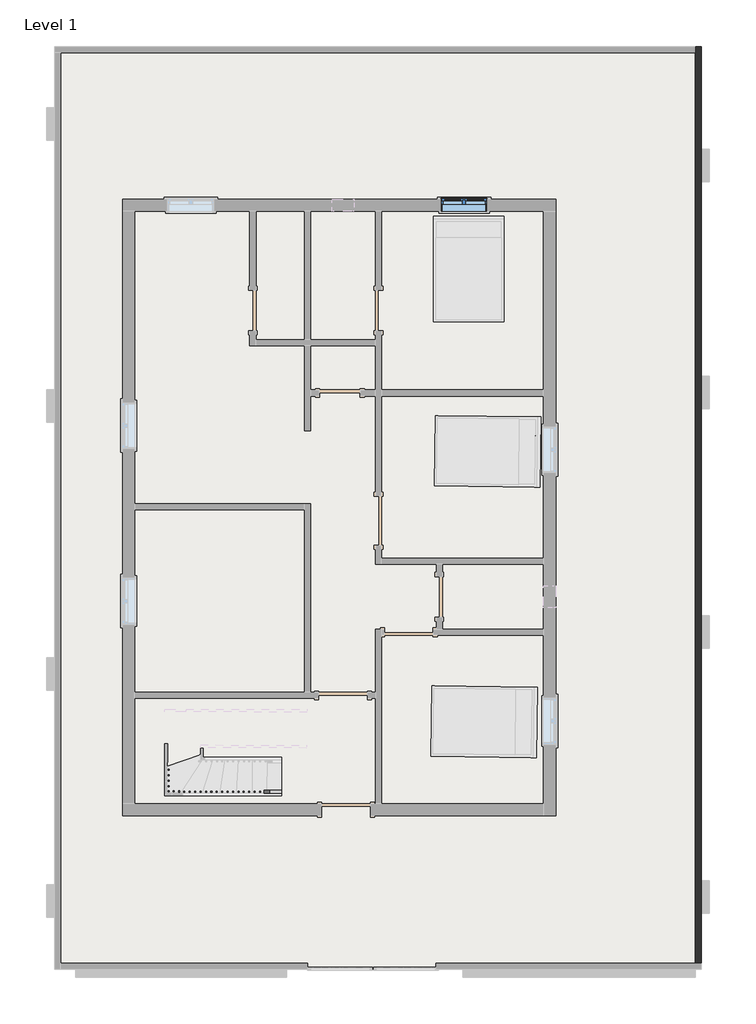
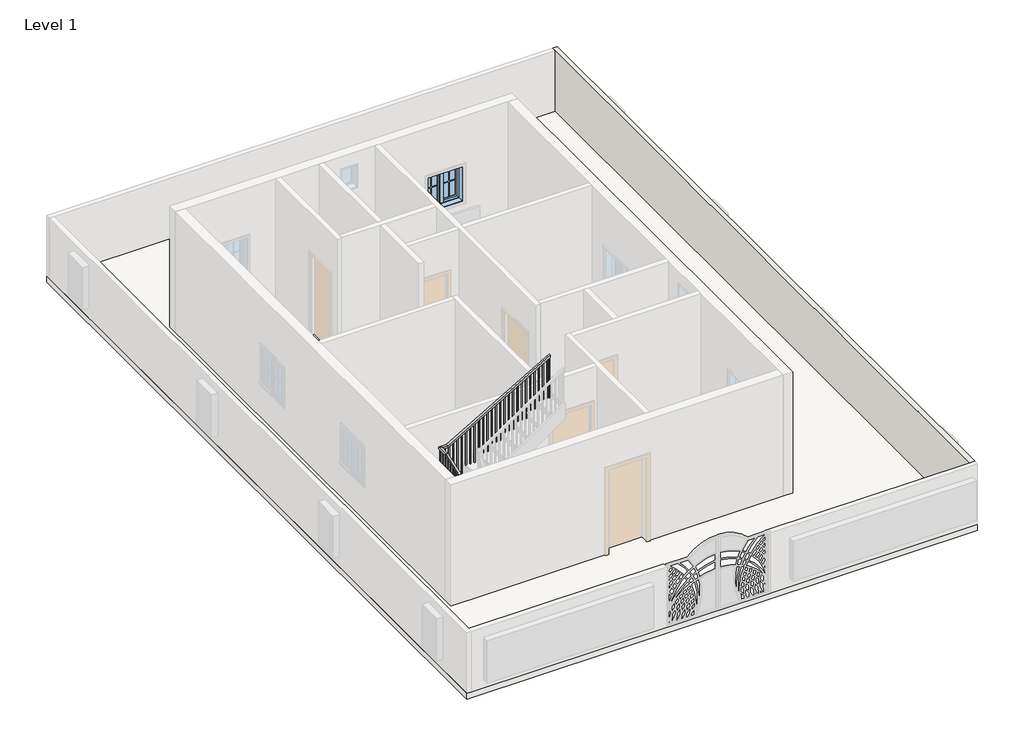
# One storey, part 2 of 3: 1 railing, 1 slab, 1 wall, 1 window.
"""IFC4 building model written with IfcOpenShell, lengths in millimetres."""

from ifc_helpers import new_model, si_unit, frame, origin, place, context, project, spatial, polyline, outline, extrude, faceted_brep, transform, mapped, element, save
from components import window_339605e1

model = new_model("IFC4")

# Units and contexts
model_context = context("Model", 3, world=origin())
ifc_project = project(units=[si_unit("LENGTHUNIT", "METRE", prefix="MILLI")], contexts=[model_context])

# Site, building, storey
site = spatial("IfcSite", under=ifc_project)
building = spatial("IfcBuilding", under=site)
storey = spatial("IfcBuildingStorey", under=building, Name="Level 1", Elevation=0.0)

# Railing
placement = place(None, origin())
element("IfcRailing", 1, ObjectType="Handrail - Rectangular", at=placement, inside=storey, context=model_context, shape_type="SolidModel", body=[
    faceted_brep([(-2342.0274141, -4826.0015756, 1083.7333333), (-2342.0274141, -4826.0015756, 1026.1375993), (-2341.8555281, -4775.2018664, 1026.1375993), (-2341.8555281, -4775.2018664, 1083.7333333), (-4375.5150225, -4819.1210645, 2170.1704289), (-4388.2346185, -4819.0780265, 2119.3704289), (-4388.0627326, -4768.2783173, 2119.3704289), (-4375.3431366, -4768.3213553, 2170.1704289), (-4491.7270905, -4818.7278493, 2170.1704289), (-4491.7270905, -4818.7278493, 2119.3704289), (-4440.7554953, -4768.100026, 2119.3704289), (-4440.7554953, -4768.100026, 2170.1704289), (-4491.153576, -4649.2296115, 2170.1704289), (-4491.1254156, -4640.9069784, 2119.3704289), (-4440.3257064, -4641.0788644, 2119.3704289), (-4440.3538668, -4649.4014974, 2170.1704289), (-4487.5712496, -3590.4977417, 2526.649629), (-4487.5430892, -3582.1751086, 2475.849629), (-4436.74338, -3582.3469946, 2475.849629), (-4436.7715404, -3590.6696276, 2526.649629), (-4486.5726753, -3295.3759891, 2526.649629), (-4486.5726753, -3295.3759891, 2475.849629), (-4435.9448521, -3346.3475843, 2475.849629), (-4435.9448521, -3346.3475843, 2526.649629), (-4306.8228358, -3295.9841909, 2526.649629), (-4292.9867911, -3296.0310065, 2475.849629), (-4293.1586771, -3346.8307157, 2475.849629), (-4306.9947217, -3346.7839001, 2526.649629), (-1866.6470501, -3304.2407725, 3962.4), (-1866.8189361, -3355.0404817, 3962.4), (-1866.8189361, -3355.0404817, 3903.4591495), (-1866.6470501, -3304.2407725, 3903.4591495)], [[[0, 1, 2, 3]], [[1, 0, 4, 5]], [[2, 1, 5, 6]], [[3, 2, 6, 7]], [[0, 3, 7, 4]], [[5, 4, 8, 9]], [[6, 5, 9, 10]], [[7, 6, 10, 11]], [[4, 7, 11, 8]], [[9, 8, 12, 13]], [[10, 9, 13, 14]], [[11, 10, 14, 15]], [[8, 11, 15, 12]], [[13, 12, 16, 17]], [[14, 13, 17, 18]], [[15, 14, 18, 19]], [[12, 15, 19, 16]], [[17, 16, 20, 21]], [[18, 17, 21, 22]], [[19, 18, 22, 23]], [[16, 19, 23, 20]], [[21, 20, 24, 25]], [[22, 21, 25, 26]], [[23, 22, 26, 27]], [[20, 23, 27, 24]], [[28, 29, 30, 31]], [[25, 24, 28, 31]], [[26, 25, 31, 30]], [[27, 26, 30, 29]], [[24, 27, 29, 28]]]),
    extrude(outline(polyline([(234.2042864, 19.05), (1221.3020607, 19.05), (1221.3020607, 0.0), (222.9957135, 0.0), (234.2042864, 19.05)])), frame((-1911.7805866, -3339.0132586, 4099.9687274), z_axis=(0.0033835818014388316, 0.9999942756707125, 0.0), x_axis=(0.0, 0.0, -1.0)), (0.0, 0.0, 1.0), 19.05),
    extrude(outline(polyline([(234.2042864, 19.0499999), (1161.5230057, 19.0499999), (1161.5230057, 0.0), (222.9957136, 0.0), (234.2042864, 19.0499999)])), frame((-2013.3800051, -3338.6694867, 4040.1896724), z_axis=(0.0033835818014388316, 0.9999942756707125, 0.0), x_axis=(0.0, 0.0, -1.0)), (0.0, 0.0, 1.0), 19.05),
    extrude(outline(polyline([(234.2042864, 19.0499999), (1101.7439506, 19.0499999), (1101.7439506, 0.0), (222.9957136, 0.0), (234.2042864, 19.0499999)])), frame((-2114.9794235, -3338.3257147, 3980.4106173), z_axis=(0.0033835818014388316, 0.9999942756707125, 0.0), x_axis=(0.0, 0.0, -1.0)), (0.0, 0.0, 1.0), 19.05),
    extrude(outline(polyline([(234.2042864, 19.0499999), (1211.2982289, 19.0499999), (1211.2982289, 0.0), (222.9957135, 0.0), (234.2042864, 19.0499999)])), frame((-2216.5788419, -3337.9819428, 3920.6315622), z_axis=(0.0033835818014388316, 0.9999942756707125, 0.0), x_axis=(0.0, 0.0, -1.0)), (0.0, 0.0, 1.0), 19.05),
    extrude(outline(polyline([(234.2042864, 19.0499999), (1151.5191739, 19.0499999), (1151.5191739, 0.0), (222.9957136, 0.0), (234.2042864, 19.0499999)])), frame((-2318.1782603, -3337.6381709, 3860.8525072), z_axis=(0.0033835818014388316, 0.9999942756707125, 0.0), x_axis=(0.0, 0.0, -1.0)), (0.0, 0.0, 1.0), 19.05),
    extrude(outline(polyline([(234.2042864, 19.0499999), (1261.0734521, 19.0499999), (1261.0734521, 0.0), (222.9957136, 0.0), (234.2042864, 19.0499999)])), frame((-2419.7776787, -3337.294399, 3801.0734521), z_axis=(0.0033835818014388316, 0.9999942756707125, 0.0), x_axis=(0.0, 0.0, -1.0)), (0.0, 0.0, 1.0), 19.05),
    extrude(outline(polyline([(234.2042864, 19.0499999), (1201.294397, 19.0499999), (1201.294397, 0.0), (222.9957136, 0.0), (234.2042864, 19.0499999)])), frame((-2521.3770971, -3336.9506271, 3741.294397), z_axis=(0.0033835818014388316, 0.9999942756707125, 0.0), x_axis=(0.0, 0.0, -1.0)), (0.0, 0.0, 1.0), 19.05),
    extrude(outline(polyline([(234.2042864, 19.05), (1141.515342, 19.05), (1141.515342, 0.0), (222.9957136, 0.0), (234.2042864, 19.05)])), frame((-2622.9765155, -3336.6068552, 3681.515342), z_axis=(0.0033835818014388316, 0.9999942756707125, 0.0), x_axis=(0.0, 0.0, -1.0)), (0.0, 0.0, 1.0), 19.05),
    extrude(outline(polyline([(234.2042864, 19.05), (1251.0696202, 19.05), (1251.0696202, 0.0), (222.9957136, 0.0), (234.2042864, 19.05)])), frame((-2724.5759339, -3336.2630833, 3621.7362869), z_axis=(0.0033835818014388316, 0.9999942756707125, 0.0), x_axis=(0.0, 0.0, -1.0)), (0.0, 0.0, 1.0), 19.05),
    extrude(outline(polyline([(234.2042864, 19.05), (1191.2905651, 19.05), (1191.2905651, 0.0), (222.9957136, 0.0), (234.2042864, 19.05)])), frame((-2826.1753523, -3335.9193114, 3561.9572318), z_axis=(0.0033835818014388316, 0.9999942756707125, 0.0), x_axis=(0.0, 0.0, -1.0)), (0.0, 0.0, 1.0), 19.05),
    extrude(outline(polyline([(234.2042865, 19.05), (1131.5115101, 19.05), (1131.5115101, 0.0), (222.9957136, 0.0), (234.2042865, 19.05)])), frame((-2927.7747707, -3335.5755395, 3502.1781768), z_axis=(0.0033835818014388316, 0.9999942756707125, 0.0), x_axis=(0.0, 0.0, -1.0)), (0.0, 0.0, 1.0), 19.05),
    extrude(outline(polyline([(234.2042864, 19.05), (1241.0657884, 19.05), (1241.0657884, 0.0), (222.9957136, 0.0), (234.2042864, 19.05)])), frame((-3029.3741891, -3335.2317675, 3442.3991217), z_axis=(0.0033835818014388316, 0.9999942756707125, 0.0), x_axis=(0.0, 0.0, -1.0)), (0.0, 0.0, 1.0), 19.05),
    extrude(outline(polyline([(234.2042864, 19.05), (1181.2867333, 19.05), (1181.2867333, 0.0), (222.9957136, 0.0), (234.2042864, 19.05)])), frame((-3130.9736075, -3334.8879956, 3382.6200666), z_axis=(0.0033835818014388316, 0.9999942756707125, 0.0), x_axis=(0.0, 0.0, -1.0)), (0.0, 0.0, 1.0), 19.05),
    extrude(outline(polyline([(234.2042865, 19.0499999), (1121.5076783, 19.0499999), (1121.5076783, 0.0), (222.9957136, 0.0), (234.2042865, 19.0499999)])), frame((-3232.573026, -3334.5442237, 3322.8410116), z_axis=(0.0033835818014388316, 0.9999942756707125, 0.0), x_axis=(0.0, 0.0, -1.0)), (0.0, 0.0, 1.0), 19.05),
    extrude(outline(polyline([(234.2042864, 19.0499999), (1231.0619565, 19.0499999), (1231.0619565, 0.0), (222.9957136, 0.0), (234.2042864, 19.0499999)])), frame((-3334.1724444, -3334.2004518, 3263.0619565), z_axis=(0.0033835818014388316, 0.9999942756707125, 0.0), x_axis=(0.0, 0.0, -1.0)), (0.0, 0.0, 1.0), 19.05),
    extrude(outline(polyline([(234.2042864, 19.0499999), (1171.2829014, 19.0499999), (1171.2829014, 0.0), (222.9957136, 0.0), (234.2042864, 19.0499999)])), frame((-3435.7718628, -3333.8566799, 3203.2829014), z_axis=(0.0033835818014388316, 0.9999942756707125, 0.0), x_axis=(0.0, 0.0, -1.0)), (0.0, 0.0, 1.0), 19.05),
    extrude(outline(polyline([(234.2042864, 19.0499999), (1111.5038463, 19.0499999), (1111.5038463, 0.0), (222.9957135, 0.0), (234.2042864, 19.0499999)])), frame((-3537.3712812, -3333.512908, 3143.5038463), z_axis=(0.0033835818014388316, 0.9999942756707125, 0.0), x_axis=(0.0, 0.0, -1.0)), (0.0, 0.0, 1.0), 19.05),
    extrude(outline(polyline([(234.2042864, 19.0499999), (1221.0581246, 19.0499999), (1221.0581246, 0.0), (222.9957136, 0.0), (234.2042864, 19.0499999)])), frame((-3638.9706996, -3333.1691361, 3083.7247913), z_axis=(0.0033835818014388316, 0.9999942756707125, 0.0), x_axis=(0.0, 0.0, -1.0)), (0.0, 0.0, 1.0), 19.05),
    extrude(outline(polyline([(234.2042864, 19.0499999), (1161.2790695, 19.0499999), (1161.2790695, 0.0), (222.9957136, 0.0), (234.2042864, 19.0499999)])), frame((-3740.570118, -3332.8253642, 3023.9457362), z_axis=(0.0033835818014388316, 0.9999942756707125, 0.0), x_axis=(0.0, 0.0, -1.0)), (0.0, 0.0, 1.0), 19.05),
    extrude(outline(polyline([(234.2042864, 19.05), (1101.5000144, 19.05), (1101.5000144, 0.0), (222.9957135, 0.0), (234.2042864, 19.05)])), frame((-3842.1695364, -3332.4815923, 2964.1666811), z_axis=(0.0033835818014388316, 0.9999942756707125, 0.0), x_axis=(0.0, 0.0, -1.0)), (0.0, 0.0, 1.0), 19.05),
    extrude(outline(polyline([(234.2042864, 19.05), (1211.0542928, 19.05), (1211.0542928, 0.0), (222.9957136, 0.0), (234.2042864, 19.05)])), frame((-3943.7689548, -3332.1378203, 2904.3876261), z_axis=(0.0033835818014388316, 0.9999942756707125, 0.0), x_axis=(0.0, 0.0, -1.0)), (0.0, 0.0, 1.0), 19.05),
    extrude(outline(polyline([(234.2042864, 19.05), (1151.2752377, 19.05), (1151.2752377, 0.0), (222.9957136, 0.0), (234.2042864, 19.05)])), frame((-4045.3683732, -3331.7940484, 2844.608571), z_axis=(0.0033835818014388316, 0.9999942756707125, 0.0), x_axis=(0.0, 0.0, -1.0)), (0.0, 0.0, 1.0), 19.05),
    extrude(outline(polyline([(234.2042864, 19.05), (1091.4961826, 19.05), (1091.4961826, 0.0), (222.9957136, 0.0), (234.2042864, 19.05)])), frame((-4146.9677916, -3331.4502765, 2784.8295159), z_axis=(0.0033835818014388316, 0.9999942756707125, 0.0), x_axis=(0.0, 0.0, -1.0)), (0.0, 0.0, 1.0), 19.05),
    extrude(outline(polyline([(234.2042865, 19.05), (1031.7171276, 19.05), (1031.7171276, 0.0), (222.9957136, 0.0), (234.2042865, 19.05)])), frame((-4248.56721, -3331.1065046, 2725.0504609), z_axis=(0.0033835818014388316, 0.9999942756707125, 0.0), x_axis=(0.0, 0.0, -1.0)), (0.0, 0.0, 1.0), 19.05),
    extrude(outline(polyline([(-4369.1520622, -3311.6483845), (-4350.1021712, -3311.7128418), (-4350.1666284, -3330.7627327), (-4369.2165194, -3330.6982755), (-4369.1520622, -3311.6483845)])), frame((0.0, 0.0, 1693.3333333), z_axis=(0.0, 0.0, 1.0), x_axis=(1.0, 0.0, 0.0)), (0.0, 0.0, 1.0), 782.5162957),
    extrude(outline(polyline([(-4470.9856602, -3380.5147968), (-4470.921203, -3361.4649058), (-4451.871312, -3361.5293631), (-4451.9357693, -3380.579254), (-4470.9856602, -3380.5147968)])), frame((0.0, 0.0, 1693.3333333), z_axis=(0.0, 0.0, 1.0), x_axis=(1.0, 0.0, 0.0)), (0.0, 0.0, 1.0), 782.5162957),
    extrude(outline(polyline([(-4471.3294321, -3482.1142152), (-4471.2649749, -3463.0643242), (-4452.215084, -3463.1287815), (-4452.2795412, -3482.1786724), (-4471.3294321, -3482.1142152)])), frame((0.0, 0.0, 1524.0), z_axis=(0.0, 0.0, 1.0), x_axis=(1.0, 0.0, 0.0)), (0.0, 0.0, 1.0), 951.849629),
    extrude(outline(polyline([(-4471.6732041, -3583.7136336), (-4471.6087468, -3564.6637426), (-4452.5588559, -3564.7281999), (-4452.6233131, -3583.7780908), (-4471.6732041, -3583.7136336)])), frame((0.0, 0.0, 1524.0), z_axis=(0.0, 0.0, 1.0), x_axis=(1.0, 0.0, 0.0)), (0.0, 0.0, 1.0), 951.849629),
    extrude(outline(polyline([(231.8070867, 19.0499999), (1148.9478489, 19.0499999), (1148.9478489, 0.0), (225.3929132, 0.0), (231.8070867, 19.0499999)])), frame((-4452.9026278, -3666.3276183, 2672.9478489), z_axis=(-0.9999942756707125, 0.003383581801438912, 0.0), x_axis=(0.0, 0.0, -1.0)), (0.0, 0.0, 1.0), 19.05),
    extrude(outline(polyline([(231.8070868, 19.0499999), (1114.7389237, 19.0499999), (1114.7389237, 0.0), (225.3929133, 0.0), (231.8070868, 19.0499999)])), frame((-4453.2463997, -3767.9270367, 2638.7389237), z_axis=(-0.9999942756707125, 0.003383581801438912, 0.0), x_axis=(0.0, 0.0, -1.0)), (0.0, 0.0, 1.0), 19.05),
    extrude(outline(polyline([(231.8070867, 19.0499999), (1080.5299984, 19.0499999), (1080.5299984, 0.0), (225.3929132, 0.0), (231.8070867, 19.0499999)])), frame((-4453.5901716, -3869.5264551, 2604.5299984), z_axis=(-0.9999942756707125, 0.003383581801438912, 0.0), x_axis=(0.0, 0.0, -1.0)), (0.0, 0.0, 1.0), 19.05),
    extrude(outline(polyline([(231.8070867, 19.05), (1215.6544064, 19.05), (1215.6544064, 0.0), (225.3929132, 0.0), (231.8070867, 19.05)])), frame((-4453.9339435, -3971.1258735, 2570.3210731), z_axis=(-0.9999942756707125, 0.003383581801438912, 0.0), x_axis=(0.0, 0.0, -1.0)), (0.0, 0.0, 1.0), 19.05),
    extrude(outline(polyline([(231.8070868, 19.05), (1181.4454812, 19.05), (1181.4454812, 0.0), (225.3929133, 0.0), (231.8070868, 19.05)])), frame((-4454.2777154, -4072.7252919, 2536.1121479), z_axis=(-0.9999942756707125, 0.003383581801438912, 0.0), x_axis=(0.0, 0.0, -1.0)), (0.0, 0.0, 1.0), 19.05),
    extrude(outline(polyline([(231.8070867, 19.05), (1147.2365559, 19.05), (1147.2365559, 0.0), (225.3929132, 0.0), (231.8070867, 19.05)])), frame((-4454.6214873, -4174.3247103, 2501.9032226), z_axis=(-0.9999942756707125, 0.003383581801438912, 0.0), x_axis=(0.0, 0.0, -1.0)), (0.0, 0.0, 1.0), 19.05),
    extrude(outline(polyline([(231.8070868, 19.05), (1113.0276307, 19.05), (1113.0276307, 0.0), (225.3929133, 0.0), (231.8070868, 19.05)])), frame((-4454.9652592, -4275.9241287, 2467.6942974), z_axis=(-0.9999942756707125, 0.003383581801438912, 0.0), x_axis=(0.0, 0.0, -1.0)), (0.0, 0.0, 1.0), 19.05),
    extrude(outline(polyline([(231.8070868, 19.05), (1248.1520388, 19.05), (1248.1520388, 0.0), (225.3929133, 0.0), (231.8070868, 19.05)])), frame((-4455.3090312, -4377.5235471, 2433.4853721), z_axis=(-0.9999942756707125, 0.003383581801438912, 0.0), x_axis=(0.0, 0.0, -1.0)), (0.0, 0.0, 1.0), 19.05),
    extrude(outline(polyline([(231.8070867, 19.05), (1213.9431135, 19.05), (1213.9431135, 0.0), (225.3929132, 0.0), (231.8070867, 19.05)])), frame((-4455.6528031, -4479.1229655, 2399.2764468), z_axis=(-0.9999942756707125, 0.003383581801438912, 0.0), x_axis=(0.0, 0.0, -1.0)), (0.0, 0.0, 1.0), 19.05),
    extrude(outline(polyline([(231.8070868, 19.0499999), (1179.7341883, 19.0499999), (1179.7341883, 0.0), (225.3929133, 0.0), (231.8070868, 19.0499999)])), frame((-4455.996575, -4580.722384, 2365.0675216), z_axis=(-0.9999942756707125, 0.003383581801438912, 0.0), x_axis=(0.0, 0.0, -1.0)), (0.0, 0.0, 1.0), 19.05),
    extrude(outline(polyline([(-4475.4546951, -4701.3072361), (-4475.3902378, -4682.2573451), (-4456.3403469, -4682.3218024), (-4456.4048041, -4701.3716933), (-4475.4546951, -4701.3072361)])), frame((0.0, 0.0, 1185.3333333), z_axis=(0.0, 0.0, 1.0), x_axis=(1.0, 0.0, 0.0)), (0.0, 0.0, 1.0), 934.0370956),
    extrude(outline(polyline([(223.5110808, 19.05), (1155.0403583, 19.05), (1155.0403583, 0.0), (233.6889192, 0.0), (223.5110808, 19.05)])), frame((-4364.4371224, -4803.2834569, 2340.3736916), z_axis=(0.0033835818014387046, 0.9999942756707125, 0.0), x_axis=(0.0, 0.0, -1.0)), (0.0, 0.0, 1.0), 19.05),
    extrude(outline(polyline([(223.5110808, 19.05), (1100.7585537, 19.05), (1100.7585537, 0.0), (233.6889192, 0.0), (223.5110808, 19.05)])), frame((-4262.837704, -4803.6272288, 2286.091887), z_axis=(0.0033835818014387046, 0.9999942756707125, 0.0), x_axis=(0.0, 0.0, -1.0)), (0.0, 0.0, 1.0), 19.05),
    extrude(outline(polyline([(223.5110808, 19.05), (1215.8100824, 19.05), (1215.8100824, 0.0), (233.6889192, 0.0), (223.5110808, 19.05)])), frame((-4161.2382856, -4803.9710007, 2231.8100824), z_axis=(0.0033835818014387046, 0.9999942756707125, 0.0), x_axis=(0.0, 0.0, -1.0)), (0.0, 0.0, 1.0), 19.05),
    extrude(outline(polyline([(223.5110809, 19.0499999), (1161.5282778, 19.0499999), (1161.5282778, 0.0), (233.6889192, 0.0), (223.5110809, 19.0499999)])), frame((-4059.6388672, -4804.3147726, 2177.5282778), z_axis=(0.0033835818014387046, 0.9999942756707125, 0.0), x_axis=(0.0, 0.0, -1.0)), (0.0, 0.0, 1.0), 19.05),
    extrude(outline(polyline([(223.5110808, 19.0499999), (1107.2464731, 19.0499999), (1107.2464731, 0.0), (233.6889191, 0.0), (223.5110808, 19.0499999)])), frame((-3958.0394488, -4804.6585445, 2123.2464731), z_axis=(0.0033835818014387046, 0.9999942756707125, 0.0), x_axis=(0.0, 0.0, -1.0)), (0.0, 0.0, 1.0), 19.05),
    extrude(outline(polyline([(223.5110808, 19.0499999), (1052.9646685, 19.0499999), (1052.9646685, 0.0), (233.6889192, 0.0), (223.5110808, 19.0499999)])), frame((-3856.4400304, -4805.0023164, 2068.9646685), z_axis=(0.0033835818014387046, 0.9999942756707125, 0.0), x_axis=(0.0, 0.0, -1.0)), (0.0, 0.0, 1.0), 19.05),
    extrude(outline(polyline([(223.5110808, 19.0499999), (1168.0161972, 19.0499999), (1168.0161972, 0.0), (233.6889192, 0.0), (223.5110808, 19.0499999)])), frame((-3754.840612, -4805.3460883, 2014.6828639), z_axis=(0.0033835818014387046, 0.9999942756707125, 0.0), x_axis=(0.0, 0.0, -1.0)), (0.0, 0.0, 1.0), 19.05),
    extrude(outline(polyline([(223.5110808, 19.0499999), (1113.7343926, 19.0499999), (1113.7343926, 0.0), (233.6889192, 0.0), (223.5110808, 19.0499999)])), frame((-3653.2411936, -4805.6898602, 1960.4010593), z_axis=(0.0033835818014387046, 0.9999942756707125, 0.0), x_axis=(0.0, 0.0, -1.0)), (0.0, 0.0, 1.0), 19.05),
    extrude(outline(polyline([(223.5110808, 19.0499999), (1059.452588, 19.0499999), (1059.452588, 0.0), (233.6889192, 0.0), (223.5110808, 19.0499999)])), frame((-3551.6417752, -4806.0336322, 1906.1192547), z_axis=(0.0033835818014387046, 0.9999942756707125, 0.0), x_axis=(0.0, 0.0, -1.0)), (0.0, 0.0, 1.0), 19.05),
    extrude(outline(polyline([(223.5110808, 19.05), (1174.5041168, 19.05), (1174.5041168, 0.0), (233.6889192, 0.0), (223.5110808, 19.05)])), frame((-3450.0423567, -4806.3774041, 1851.8374501), z_axis=(0.0033835818014387046, 0.9999942756707125, 0.0), x_axis=(0.0, 0.0, -1.0)), (0.0, 0.0, 1.0), 19.05),
    extrude(outline(polyline([(223.5110809, 19.05), (1120.2223122, 19.05), (1120.2223122, 0.0), (233.6889192, 0.0), (223.5110809, 19.05)])), frame((-3348.4429383, -4806.721176, 1797.5556455), z_axis=(0.0033835818014387046, 0.9999942756707125, 0.0), x_axis=(0.0, 0.0, -1.0)), (0.0, 0.0, 1.0), 19.05),
    extrude(outline(polyline([(223.5110808, 19.05), (1065.9405075, 19.05), (1065.9405075, 0.0), (233.6889191, 0.0), (223.5110808, 19.05)])), frame((-3246.8435199, -4807.0649479, 1743.2738408), z_axis=(0.0033835818014387046, 0.9999942756707125, 0.0), x_axis=(0.0, 0.0, -1.0)), (0.0, 0.0, 1.0), 19.05),
    extrude(outline(polyline([(223.5110808, 19.05), (1180.9920362, 19.05), (1180.9920362, 0.0), (233.6889192, 0.0), (223.5110808, 19.05)])), frame((-3145.2441015, -4807.4087198, 1688.9920362), z_axis=(0.0033835818014387046, 0.9999942756707125, 0.0), x_axis=(0.0, 0.0, -1.0)), (0.0, 0.0, 1.0), 19.05),
    extrude(outline(polyline([(223.5110808, 19.05), (1126.7102316, 19.05), (1126.7102316, 0.0), (233.6889192, 0.0), (223.5110808, 19.05)])), frame((-3043.6446831, -4807.7524917, 1634.7102316), z_axis=(0.0033835818014387046, 0.9999942756707125, 0.0), x_axis=(0.0, 0.0, -1.0)), (0.0, 0.0, 1.0), 19.05),
    extrude(outline(polyline([(223.5110808, 19.05), (1072.428427, 19.05), (1072.428427, 0.0), (233.6889192, 0.0), (223.5110808, 19.05)])), frame((-2942.0452647, -4808.0962636, 1580.428427), z_axis=(0.0033835818014387046, 0.9999942756707125, 0.0), x_axis=(0.0, 0.0, -1.0)), (0.0, 0.0, 1.0), 19.05),
    extrude(outline(polyline([(223.5110808, 19.05), (1187.4799557, 19.05), (1187.4799557, 0.0), (233.6889192, 0.0), (223.5110808, 19.05)])), frame((-2840.4458463, -4808.4400355, 1526.1466224), z_axis=(0.0033835818014387046, 0.9999942756707125, 0.0), x_axis=(0.0, 0.0, -1.0)), (0.0, 0.0, 1.0), 19.05),
    extrude(outline(polyline([(223.5110809, 19.0499999), (1133.1981511, 19.0499999), (1133.1981511, 0.0), (233.6889192, 0.0), (223.5110809, 19.0499999)])), frame((-2738.8464279, -4808.7838074, 1471.8648178), z_axis=(0.0033835818014387046, 0.9999942756707125, 0.0), x_axis=(0.0, 0.0, -1.0)), (0.0, 0.0, 1.0), 19.05),
    extrude(outline(polyline([(223.5110809, 19.0499999), (1078.9163465, 19.0499999), (1078.9163465, 0.0), (233.6889192, 0.0), (223.5110809, 19.0499999)])), frame((-2637.2470095, -4809.1275794, 1417.5830132), z_axis=(0.0033835818014387046, 0.9999942756707125, 0.0), x_axis=(0.0, 0.0, -1.0)), (0.0, 0.0, 1.0), 19.05),
    extrude(outline(polyline([(223.5110808, 19.0499999), (1193.9678752, 19.0499999), (1193.9678752, 0.0), (233.6889191, 0.0), (223.5110808, 19.0499999)])), frame((-2535.6475911, -4809.4713513, 1363.3012085), z_axis=(0.0033835818014387046, 0.9999942756707125, 0.0), x_axis=(0.0, 0.0, -1.0)), (0.0, 0.0, 1.0), 19.05),
    extrude(outline(polyline([(223.5110808, 19.0499999), (1139.6860706, 19.0499999), (1139.6860706, 0.0), (233.6889192, 0.0), (223.5110808, 19.0499999)])), frame((-2434.0481727, -4809.8151232, 1309.0194039), z_axis=(0.0033835818014387046, 0.9999942756707125, 0.0), x_axis=(0.0, 0.0, -1.0)), (0.0, 0.0, 1.0), 19.05),
    extrude(outline(polyline([(-4470.8159378, -3330.3545036), (-4470.7514806, -3311.3046126), (-4451.7015896, -3311.3690698), (-4451.7660469, -3330.4189608), (-4470.8159378, -3330.3545036)])), frame((0.0, 0.0, 1693.3333333), z_axis=(0.0, 0.0, 1.0), x_axis=(1.0, 0.0, 0.0)), (0.0, 0.0, 1.0), 782.5162957),
    extrude(outline(polyline([(-4456.748576, -4802.9711117), (-4475.798467, -4802.9066545), (-4475.7340098, -4783.8567635), (-4456.6841188, -4783.9212208), (-4456.748576, -4802.9711117)])), frame((0.0, 0.0, 1185.3333333), z_axis=(0.0, 0.0, 1.0), x_axis=(1.0, 0.0, 0.0)), (0.0, 0.0, 1.0), 934.0370956),
    extrude(outline(polyline([(234.2042864, 19.05), (1247.7881964, 19.05), (1247.7881964, 0.0), (222.9957136, 0.0), (234.2042864, 19.05)])), frame((-1866.7652217, -3339.1655726, 4126.4548631), z_axis=(0.0033835818014388316, 0.9999942756707125, 0.0), x_axis=(0.0, 0.0, -1.0)), (0.0, 0.0, 1.0), 19.05),
    extrude(outline(polyline([(223.5656878, 19.05), (1090.5752441, 19.05), (1090.5752441, 0.0), (233.6343122, 0.0), (223.5656878, 19.05)])), frame((-2341.9736997, -4810.1266665, 1259.9085774), z_axis=(0.0033835818014387046, 0.9999942756707125, 0.0), x_axis=(0.0, 0.0, -1.0)), (0.0, 0.0, 1.0), 19.05),
])

# Slab
element("IfcSlab", 2, ObjectType="Generic - 12\"", at=placement, inside=storey, context=model_context, shape_type="SweptSolid", body=[
    extrude(outline(polyline([(5544.7022658, 9200.5938411), (5544.7022658, -8134.9061589), (-6609.1977342, -8134.9061589), (-6609.1977342, 9200.5938411), (5544.7022658, 9200.5938411)])), frame((0.0, 0.0, -152.4), z_axis=(0.0, 0.0, 1.0), x_axis=(1.0, 0.0, 0.0)), (0.0, 0.0, 1.0), 152.4),
])

# Wall
element("IfcWall", 3, ObjectType="wall4.5\"", at=placement, inside=storey, context=model_context, shape_type="Brep", body=[
    faceted_brep([(5430.4022658, 9200.5938411, 0.0), (5430.4022658, 9086.2938411, 0.0), (5430.4022658, -8020.6061589, 0.0), (5430.4022658, -8020.6061589, 1524.0), (5430.4022658, 9086.2938411, 1524.0), (5430.4022658, 9200.5938411, 1524.0), (5544.7022658, 9200.5938411, 0.0), (5544.7022658, 9200.5938411, 1524.0), (5544.7022658, -8020.6061589, 1524.0), (5544.7022658, -8020.6061589, 0.0)], [[[0, 1, 2, 3, 4, 5]], [[6, 7, 8, 9]], [[2, 1, 0, 6, 9]], [[5, 4, 3, 8, 7]], [[0, 5, 7, 6]], [[3, 2, 9, 8]]]),
])

# Window
window_shape = window_339605e1(model_context)
element("IfcWindow", 4, ObjectType="Window-Casement-Double : 34\" x 36\"", at=placement, inside=storey, context=model_context, shape_type="MappedRepresentation", body=[
    mapped(window_shape, transform((1088.0382686, 6216.8821212, 0.0), x_axis=(1.0, 0.0, 0.0), y_axis=(0.0, 1.0, 0.0), z_axis=(0.0, 0.0, 1.0))),
])

save(model, "model.ifc")

# Revit data of these elements
# Type "Handrail - Rectangular"
#   Assembly Code = "C2010400"
#   built-in parameter 1008612 = 0.0416667 (stored number, unit not read)
#   built-in parameter 1008611 = 0.0416667 (stored number, unit not read)
#   built-in parameter 1008609 = 0.333333 (stored number, unit not read)
#   built-in parameter 1008604 = 0.166667 (stored number, unit not read)
#   built-in parameter 1008603 = 0.166667 (stored number, unit not read)
#   Railing Height = 3' - 0"
#   built-in parameter 1008630 = 2
#   built-in parameter 1008610 = 2
#   built-in parameter 1008618 = Baluster - Square : 3/4"
# Type "Generic - 12\""
#   Assembly Code = "B1010"
#   Function = 0
#   Layers, outside or top first: 0' - 6" no material (function 1)
# Type "wall4.5\""
#   Assembly Code = "B2010"
#   Layers, outside or top first: 0' - 4 1/2" no material (function 1)
# Type "Window-Casement-Double : 34\" x 36\""
#   Type Mark = "14"
#   Fire Rating = "0.5h"
#   Assembly Code = "B2020100"
#   Analytic Construction = "Double glazing - domestic"
#   Frame Extension [instance default] = 0' - 0 1/4"
#   Window Inset [instance default] = 0' - 0"
#   Wall Thickness [instance default] = 0' - 6"
#   Interior Wall Closure [instance default] = 0' - 2 1/4"
#   Half Width = 1' - 5"
#   Visual Light Transmittance = 0.81
#   Thermal Resistance (R) = 1.8146 (h·ft²·°F)/BTU
#   Solar Heat Gain Coefficient = 0.76
#   Rough Width = 2' - 10 1/2"
#   Rough Height = 3' - 0 1/2"
#   Height = 3' - 0"
#   Heat Transfer Coefficient (U) = 0.5511 BTU/(h·ft²·°F)
#   Exterior Wall Closure [instance default] = 0' - 1 1/4"
#   Extension Jamb [instance default] = 0' - 2 1/4"
#   Default Sill Height = 3' - 0"
#   Width = 2' - 10"
#   Define Thermal Properties by = 0
#   Muntin Visibility = yes
#   Interior Trim Visibility [instance default] = yes
#   Exterior Trim Visibility [instance default] = yes
#   Extension Jamb Visibility [instance default] = yes
#   Interior Trim Material = Wood - Stained
#   Muntin Pattern = Muntin Pattern_2x2 : Muntin Pattern_2x2
#   Interior Trim = Trim-Window-Interior-Flat : Picture Frame
#   Interior Frame Material = Wood - Stained
#   Glass Panel Material = Glass
#   Exterior Trim Material = Clad - White
#   Exterior Trim = Trim-Window-Exterior-Flat : with Sill
#   Exterior Frame Material = Clad - White
#   Wall Closure = (empty or 0)
# Element 1 (IfcRailing, "Handrail - Rectangular")
#   Phase Created = New Construction
# Element 2 (IfcSlab, "Generic - 12\"")
#   Height Offset From Level = 0' - 0"
#   Phase Created = New Construction
#   Materials on its faces: "Default Floor"
# Element 3 (IfcWall, "wall4.5\"")
#   Top Offset = 0' - 0"
#   Base Offset = 0' - 0"
#   Unconnected Height = 5' - 0"
#   wall height = 5' - 0"
#   Phase Created = New Construction
#   Base Constraint = Level 1
#   Materials on its faces: "Default Wall", "Door - Frame"
# Element 4 (IfcWindow, "Window-Casement-Double : 34\" x 36\"")
#   Mark = "3"
#   Window Inset = 0' - 0"
#   Interior Wall Closure = 0' - 2 1/4"
#   Frame Extension = 0' - 0 1/4"
#   Exterior Wall Closure = 0' - 1 1/4"
#   Interior Trim Visibility = yes
#   Exterior Trim Visibility = yes
#   Phase Created = New Construction
#   Materials on its faces: "Wood - Stained", "Glass", "Clad - White"
# Materials
#   "Wood - Stained": class "Wood", colour RGB 224 178 126, transparency 0, Cost = 0
#   "Glass": class "Glass", colour RGB 0 128 192, transparency 0.75, Description = "Soda Lime Glass", Cost = 0
#   "Clad - White": class "Wood", colour RGB 242 242 238, transparency 0, Cost = 0
#   "Default Floor": colour RGB 128 128 128, transparency 0, Cost = 0
#   "Default Wall": colour RGB 128 128 128, transparency 0, Cost = 0
#   "Door - Frame": colour RGB 118 70 51, transparency 0, Cost = 0
